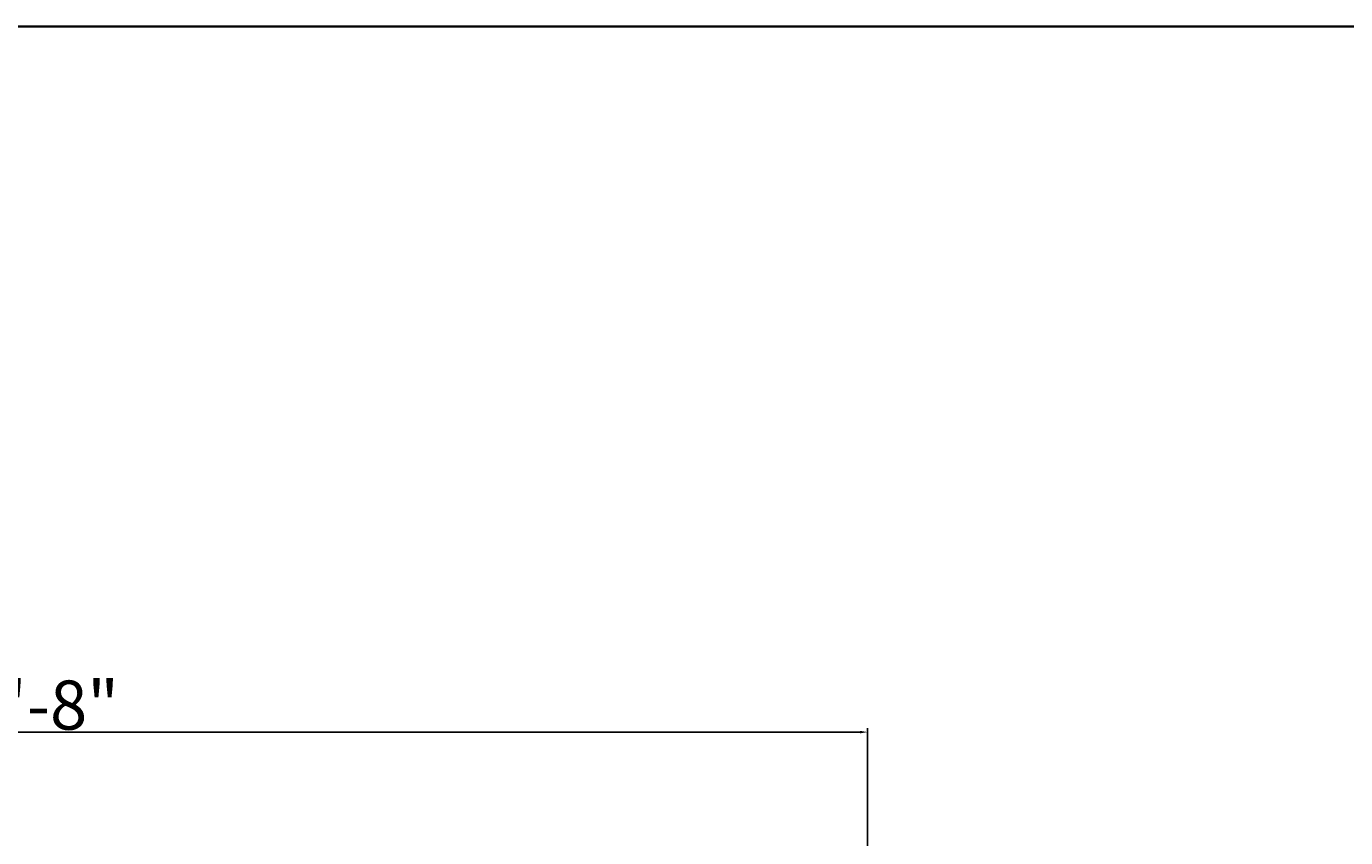
# Model space of a CAD drawing. Units: inches. Extents: x -31485 to -28799, y 18003 to 19130.
# Tile 7 of 15: x -30936 to -30506, y 18866 to 19130. Entities that reach past the tile are written whole.
import ezdxf

# ---------------------------------------------------------------- set-up
doc = ezdxf.new("R2010")
doc.units = ezdxf.units.IN
doc.layers.add('A-ANNO-DIMS', color=2, linetype='Continuous', lineweight=18)
doc.layers.add('A-ANNO-TTLB', color=7, linetype='Continuous', lineweight=35)
doc.styles.get("Standard").update_dxf_attribs({"font": 'arial.ttf'})
doc.dimstyles.new('ISO-25', dxfattribs={"dimtxt": 2.5, "dimasz": 2.5, "dimexe": 1.25, "dimexo": 0.625, "dimtad": 1, "dimdec": 0, "dimlunit": 3, "dimtxsty": 'Standard', "dimcen": 2.5, "dimadec": 0, "dimazin": 0, "dimtfac": 1, "dimtdec": 0, "dimtmove": 0, "dimatfit": 3, "dimfxl": 1, "dimarcsym": 0})

# ---------------------------------------------------------------- blocks, each defined once
blk = doc.blocks.new('*D200')
at = {"layer": 'A-ANNO-DIMS', "color": 0, "lineweight": -2, "transparency": 16777216}
for p, q in [((-31209.53, 18824.43), (-31209.53, 18901.41)), ((-31207.03, 18900.16), (-30664.03, 18900.16)), ((-30661.53, 18824.43), (-30661.53, 18901.41))]:
    blk.add_line(p, q, dxfattribs=at)
at = {"layer": 'A-ANNO-DIMS', "color": 0, "transparency": 16777216}
for points in [[(-31207.03, 18900.58), (-31207.03, 18899.75), (-31209.53, 18900.16)], [(-30664.03, 18900.58), (-30664.03, 18899.75), (-30661.53, 18900.16)]]:
    blk.add_solid(points, dxfattribs=at)
at = {"layer": 'Defpoints', "color": 0, "transparency": 16777216}
for p in [(-30661.53, 18900.16), (-31209.53, 18823.8), (-30661.53, 18823.8)]:
    blk.add_point(p, dxfattribs=at)
at = {"layer": 'A-ANNO-DIMS', "color": 0, "transparency": 16777216, "insert": (-30935.53, 18908.96), "char_height": 2.5, "attachment_point": 5}
blk.add_mtext('{\\H6.4x;45\'-8"}', dxfattribs=at)

msp = doc.modelspace()

# ---------------------------------------------------------------- linework, layer by layer
at = {"layer": 'A-ANNO-TTLB'}
msp.add_lwpolyline([(-31485.1, 19129.94), (-28798.64, 19129.94), (-28798.64, 18002.86), (-31485.1, 18002.86)], close=True, dxfattribs=at)

# ---------------------------------------------------------------- dimensions: what is measured, and where the dimension line sits
at = {"layer": 'A-ANNO-DIMS'}
dim = msp.add_linear_dim(base=(-30661.53, 18900.16), p1=(-31209.53, 18823.8), p2=(-30661.53, 18823.8), text='{\\H6.4x;<>}', dimstyle='ISO-25', override={"dimclrd": 0, "dimclre": 0, "dimclrt": 0}, dxfattribs=at)
dim.commit()
dim.dimension.update_dxf_attribs({"geometry": '*D200', "text_midpoint": (-30935.53, 18908.96)})

doc.saveas('drawing.dxf')
